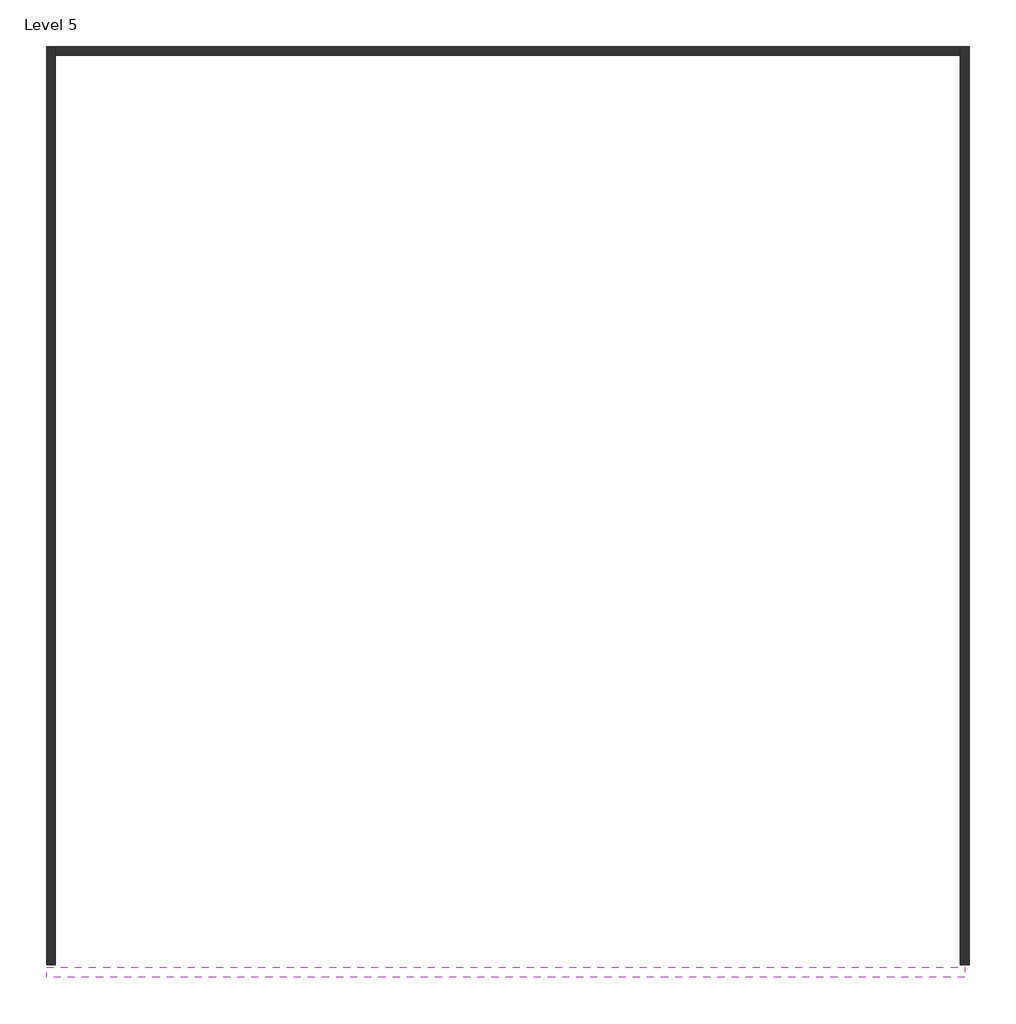
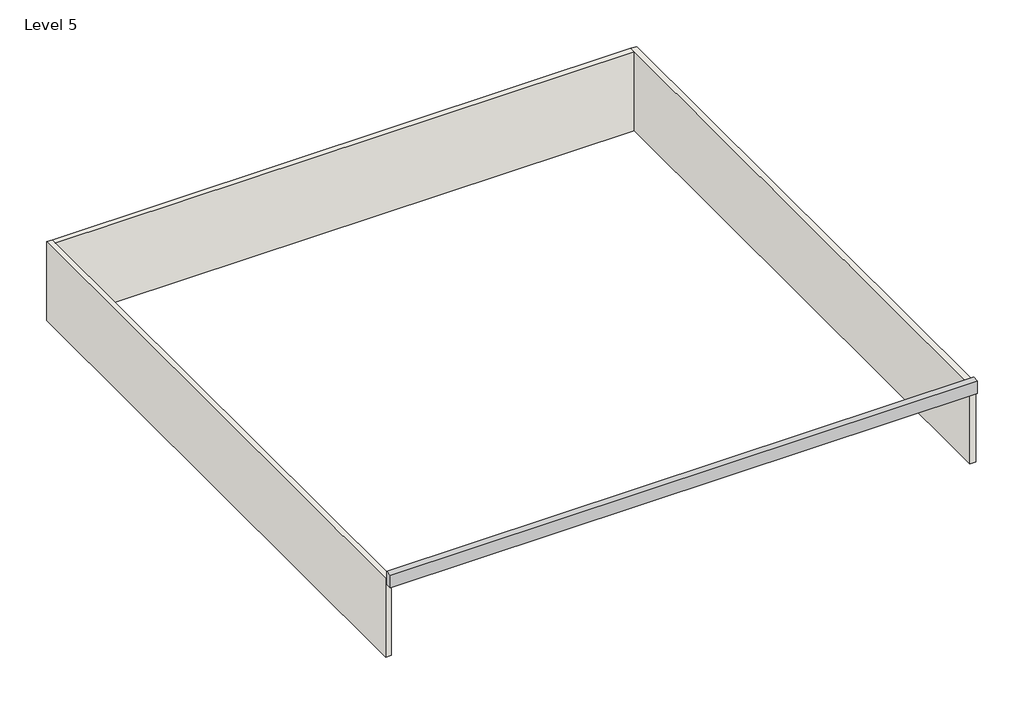
# One storey: 3 walls, 1 proxy.
"""IFC4 building model written with IfcOpenShell, lengths in millimetres."""

from ifc_helpers import new_model, si_unit, frame, origin, place, context, project, spatial, polyline, outline, extrude, faceted_brep, transform, mapped, element, save
from components import generic_models_5_generic_models_5_c0e4cdeb

model = new_model("IFC4")

# Units and contexts
model_context = context("Model", 3, world=origin())
ifc_project = project(units=[si_unit("LENGTHUNIT", "METRE", prefix="MILLI")], contexts=[model_context])

# Site, building, storey
site = spatial("IfcSite", under=ifc_project)
building = spatial("IfcBuilding", under=site)
storey = spatial("IfcBuildingStorey", under=building, Name="Level 5", Elevation=6553.2)

# Proxy
placement = place(None, origin())
generic_models_5_generic_models_5_shape = generic_models_5_generic_models_5_c0e4cdeb(model_context)
element("IfcBuildingElementProxy", 1, Name="Generic Models 5 : Generic Models 5", ObjectType="Generic Models 5 : Generic Models 5", at=placement, inside=storey, context=model_context, shape_type="MappedRepresentation", body=[
    mapped(generic_models_5_generic_models_5_shape, transform((0.0, 0.0, 0.0), x_axis=(1.0, 0.0, 0.0), y_axis=(0.0, 1.0, 0.0), z_axis=(0.0, 0.0, 1.0))),
])

# Walls
element("IfcWall", 2, ObjectType="outer wall", at=placement, inside=storey, context=model_context, shape_type="Brep", body=[
    faceted_brep([(-8731.5629849, -3682.5004242, 6553.2), (-8731.5629849, 17551.8995758, 6553.2), (-8731.5629849, 17755.0995758, 6553.2), (-8731.5629849, 17755.0995758, 9601.2), (-8731.5629849, 17551.8995758, 9601.2), (-8731.5629849, -3682.5004242, 9601.2), (-8934.7629849, -3682.5004242, 6553.2), (-8934.7629849, -3682.5004242, 9601.2), (-8934.7629849, 17755.0995758, 9601.2), (-8934.7629849, 17755.0995758, 6553.2)], [[[0, 1, 2, 3, 4, 5]], [[6, 7, 8, 9]], [[2, 1, 0, 6, 9]], [[0, 5, 7, 6]], [[5, 4, 3, 8, 7]], [[3, 2, 9, 8]]]),
])
element("IfcWall", 3, ObjectType="outer wall", at=placement, inside=storey, context=model_context, shape_type="Brep", body=[
    faceted_brep([(12604.4370151, -3682.5004242, 6553.2), (12604.4370151, 17755.0995758, 6553.2), (12604.4370151, 17755.0995758, 9601.2), (12604.4370151, -3682.5004242, 9601.2), (12401.2370151, -3682.5004242, 6553.2), (12401.2370151, -3682.5004242, 9601.2), (12401.2370151, 17551.8995758, 9601.2), (12401.2370151, 17755.0995758, 9601.2), (12401.2370151, 17755.0995758, 6553.2), (12401.2370151, 17551.8995758, 6553.2)], [[[0, 1, 2, 3]], [[4, 5, 6, 7, 8, 9]], [[1, 0, 4, 9, 8]], [[0, 3, 5, 4]], [[3, 2, 7, 6, 5]], [[2, 1, 8, 7]]]),
])
element("IfcWall", 4, ObjectType="outer wall", at=placement, inside=storey, context=model_context, shape_type="SweptSolid", body=[
    extrude(outline(polyline([(12401.2370151, 17551.8995758), (-8731.5629849, 17551.8995758), (-8731.5629849, 17755.0995758), (12401.2370151, 17755.0995758), (12401.2370151, 17551.8995758)])), frame((0.0, 0.0, 6553.2), z_axis=(0.0, 0.0, 1.0), x_axis=(1.0, 0.0, 0.0)), (0.0, 0.0, 1.0), 3048.0),
])

save(model, "model.ifc")

# Revit data of these elements
# Type "outer wall"
#   Assembly Code = "B2010"
#   Layers, outside or top first: 0' - 8" "Copper" (function 1)
# Element 1 (IfcBuildingElementProxy, "Generic Models 5 : Generic Models 5")
#   Phase Created = New Construction
# Elements 2, 3, 4 (IfcWall, "outer wall")
#   Top Offset = 0' - 0"
#   Base Offset = 0' - 0"
#   Unconnected Height = 10' - 0"
#   wall height = 10' - 0"
#   Phase Created = New Construction
#   Base Constraint = Level 5
#   Materials on its faces: "Copper"
# Materials
#   "Copper": class "Metal", colour RGB 0 0 0, transparency 0, Description = "Copper, matte finish", Cost = 0
